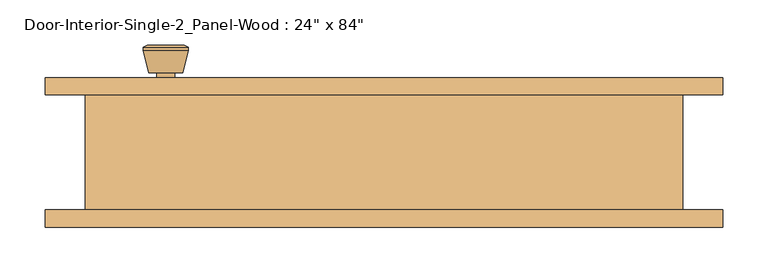
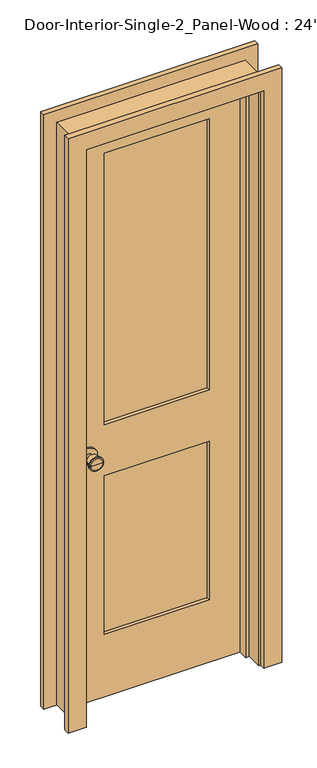
"""IFC4 building model written with IfcOpenShell, lengths in millimetres: door geometry."""

from ifc_helpers import new_model, si_unit, point, frame, frame_2d, origin, place, context, project, spatial, polyline, circle_curve, trimmed, segment, composite_curve, outline, extrude, faceted_brep, source, transform, mapped, element, save
from ifc_brep_helpers import plane_surface, cylinder_surface, revolved_surface, advanced_brep


def door_596d7c92(model_context):
    return source(origin(), model_context, "Body", "SolidModel", [
        advanced_brep(
        [(-241.3, 19.4, 914.4), (-231.3, 19.4, 914.4), (-251.3, 19.4, 914.4), (-220.8241324, -29.6, 914.4), (-241.3, -29.6, 914.4), (-261.7758676, -29.6, 914.4), (-216.3, -27.7721319, 914.4), (-266.3, -27.7721319, 914.4), (-216.3, -24.3084537, 914.4), (-266.3, -24.3084537, 914.4), (-222.663764, 0.4, 914.4), (-259.936236, 0.4, 914.4), (-231.3, 0.4, 914.4), (-251.3, 0.4, 914.4)],
        [
            (0, 1),
            (1, 2, circle_curve(frame((-241.3, 19.4, 914.4), z_axis=(0.0, 1.0, 0.0), x_axis=(-1.0, 0.0, 0.0)), 10.0)),
            (2, 0),
            (2, 1, circle_curve(frame((-241.3, 19.4, 914.4), z_axis=(0.0, 1.0, 0.0), x_axis=(-1.0, 0.0, 0.0)), 10.0)),
            (3, 4),
            (4, 5),
            (5, 3, circle_curve(frame((-241.3, -29.6, 914.4), z_axis=(0.0, -1.0, 0.0), x_axis=(-1.0, 0.0, 0.0)), 20.4758676)),
            (3, 5, circle_curve(frame((-241.3, -29.6, 914.4), z_axis=(0.0, -1.0, 0.0), x_axis=(-1.0, 0.0, 0.0)), 20.4758676)),
            (6, 3),
            (5, 7),
            (7, 6, circle_curve(frame((-241.3, -27.7721319, 914.4), z_axis=(0.0, -1.0, 0.0), x_axis=(-1.0, 0.0, 0.0)), 25.0)),
            (6, 7, circle_curve(frame((-241.3, -27.7721319, 914.4), z_axis=(0.0, -1.0, 0.0), x_axis=(-1.0, 0.0, 0.0)), 25.0)),
            (8, 6),
            (7, 9),
            (9, 8, circle_curve(frame((-241.3, -24.3084537, 914.4), z_axis=(0.0, -1.0, 0.0), x_axis=(-1.0, 0.0, 0.0)), 25.0)),
            (8, 9, circle_curve(frame((-241.3, -24.3084537, 914.4), z_axis=(0.0, -1.0, 0.0), x_axis=(-1.0, 0.0, 0.0)), 25.0)),
            (10, 8),
            (9, 11),
            (11, 10, circle_curve(frame((-241.3, 0.4, 914.4), z_axis=(0.0, -1.0, 0.0), x_axis=(-1.0, 0.0, 0.0)), 18.636236)),
            (10, 11, circle_curve(frame((-241.3, 0.4, 914.4), z_axis=(0.0, -1.0, 0.0), x_axis=(-1.0, 0.0, 0.0)), 18.636236)),
            (12, 10),
            (11, 13),
            (13, 12, circle_curve(frame((-241.3, 0.4, 914.4), z_axis=(0.0, -1.0, 0.0), x_axis=(-1.0, 0.0, 0.0)), 10.0)),
            (12, 13, circle_curve(frame((-241.3, 0.4, 914.4), z_axis=(0.0, -1.0, 0.0), x_axis=(-1.0, 0.0, 0.0)), 10.0)),
            (1, 12),
            (13, 2),
        ],
        [
            plane_surface(frame((-241.3, 19.4, 914.4), z_axis=(0.0, 1.0, 0.0), x_axis=(-1.0, 0.0, 0.0))),
            plane_surface(frame((-241.3, -29.6, 914.4), z_axis=(0.0, -1.0, 0.0), x_axis=(-1.0, 0.0, 0.0))),
            revolved_surface(polyline([(-261.7758676, -29.6, 914.4), (-266.3, -27.7721319, 914.4)]), (-241.3, 19.4, 914.4), (0.0, 1.0, 0.0)),
            cylinder_surface(frame((-241.3, 19.4, 914.4), z_axis=(0.0, 1.0, 0.0), x_axis=(-1.0, 0.0, 0.0)), 25.0),
            revolved_surface(polyline([(-266.3, -24.3084537, 914.4), (-259.936236, 0.4, 914.4)]), (-241.3, 19.4, 914.4), (0.0, 1.0, 0.0)),
            plane_surface(frame((-241.3, 0.4, 914.4), z_axis=(0.0, 1.0, 0.0), x_axis=(-1.0, 0.0, 0.0))),
            cylinder_surface(frame((-241.3, 19.4, 914.4), z_axis=(0.0, 1.0, 0.0), x_axis=(-1.0, 0.0, 0.0)), 10.0),
        ],
        [
            (0, [[1, 2, 3]]),
            (0, [[-3, 4, -1]]),
            (1, [[5, 6, 7]]),
            (1, [[-6, -5, 8]]),
            (2, [[9, -7, 10, 11]]),
            (2, [[-10, -8, -9, 12]]),
            (3, [[13, -11, 14, 15]]),
            (3, [[-14, -12, -13, 16]]),
            (4, [[17, -15, 18, 19]]),
            (4, [[-18, -16, -17, 20]]),
            (5, [[21, -19, 22, 23]]),
            (5, [[-22, -20, -21, 24]]),
            (6, [[25, -23, 26, -2]]),
            (6, [[-26, -24, -25, -4]]),
        ],
    ),
        extrude(outline(composite_curve([segment(trimmed(circle_curve(frame_2d((914.4, -241.3)), 30.0), [point((914.4, -271.3))], [point((914.4, -211.3))], False, "CARTESIAN"), True, "CONTINUOUS"), segment(trimmed(circle_curve(frame_2d((914.4, -241.3)), 30.0), [point((914.4, -211.3))], [point((914.4, -271.3))], False, "CARTESIAN"), True, "CONTINUOUS")], self_intersect=False)), frame((0.0, 19.4, 0.0), z_axis=(0.0, 1.0, 0.0), x_axis=(0.0, 0.0, 1.0)), (0.0, 0.0, 1.0), 6.0),
        advanced_brep(
        [(-241.3, 66.325, 914.4), (-251.3, 66.325, 914.4), (-231.3, 66.325, 914.4), (-220.8241324, 115.325, 914.4), (-261.7758676, 115.325, 914.4), (-241.3, 115.325, 914.4), (-216.3, 113.4971319, 914.4), (-266.3, 113.4971319, 914.4), (-216.3, 110.0334537, 914.4), (-266.3, 110.0334537, 914.4), (-222.663764, 85.325, 914.4), (-259.936236, 85.325, 914.4), (-231.3, 85.325, 914.4), (-251.3, 85.325, 914.4)],
        [
            (0, 1),
            (1, 2, circle_curve(frame((-241.3, 66.325, 914.4), z_axis=(0.0, -1.0, 0.0), x_axis=(-1.0, 0.0, 0.0)), 10.0)),
            (2, 0),
            (2, 1, circle_curve(frame((-241.3, 66.325, 914.4), z_axis=(0.0, -1.0, 0.0), x_axis=(-1.0, 0.0, 0.0)), 10.0)),
            (3, 4, circle_curve(frame((-241.3, 115.325, 914.4), z_axis=(0.0, 1.0, 0.0), x_axis=(-1.0, 0.0, 0.0)), 20.4758676)),
            (4, 5),
            (5, 3),
            (4, 3, circle_curve(frame((-241.3, 115.325, 914.4), z_axis=(0.0, 1.0, 0.0), x_axis=(-1.0, 0.0, 0.0)), 20.4758676)),
            (6, 7, circle_curve(frame((-241.3, 113.4971319, 914.4), z_axis=(0.0, 1.0, 0.0), x_axis=(-1.0, 0.0, 0.0)), 25.0)),
            (7, 4),
            (3, 6),
            (7, 6, circle_curve(frame((-241.3, 113.4971319, 914.4), z_axis=(0.0, 1.0, 0.0), x_axis=(-1.0, 0.0, 0.0)), 25.0)),
            (8, 9, circle_curve(frame((-241.3, 110.0334537, 914.4), z_axis=(0.0, 1.0, 0.0), x_axis=(-1.0, 0.0, 0.0)), 25.0)),
            (9, 7),
            (6, 8),
            (9, 8, circle_curve(frame((-241.3, 110.0334537, 914.4), z_axis=(0.0, 1.0, 0.0), x_axis=(-1.0, 0.0, 0.0)), 25.0)),
            (10, 11, circle_curve(frame((-241.3, 85.325, 914.4), z_axis=(0.0, 1.0, 0.0), x_axis=(-1.0, 0.0, 0.0)), 18.636236)),
            (11, 9),
            (8, 10),
            (11, 10, circle_curve(frame((-241.3, 85.325, 914.4), z_axis=(0.0, 1.0, 0.0), x_axis=(-1.0, 0.0, 0.0)), 18.636236)),
            (12, 13, circle_curve(frame((-241.3, 85.325, 914.4), z_axis=(0.0, 1.0, 0.0), x_axis=(-1.0, 0.0, 0.0)), 10.0)),
            (13, 11),
            (10, 12),
            (13, 12, circle_curve(frame((-241.3, 85.325, 914.4), z_axis=(0.0, 1.0, 0.0), x_axis=(-1.0, 0.0, 0.0)), 10.0)),
            (1, 13),
            (12, 2),
        ],
        [
            plane_surface(frame((-241.3, 66.325, 914.4), z_axis=(0.0, -1.0, 0.0), x_axis=(-1.0, 0.0, 0.0))),
            plane_surface(frame((-241.3, 115.325, 914.4), z_axis=(0.0, 1.0, 0.0), x_axis=(-1.0, 0.0, 0.0))),
            revolved_surface(polyline([(-261.7758676, 115.325, 914.4), (-266.3, 113.4971319, 914.4)]), (-241.3, 66.325, 914.4), (0.0, -1.0, 0.0)),
            cylinder_surface(frame((-241.3, 66.325, 914.4), z_axis=(0.0, -1.0, 0.0), x_axis=(-1.0, 0.0, 0.0)), 25.0),
            revolved_surface(polyline([(-266.3, 110.0334537, 914.4), (-259.936236, 85.325, 914.4)]), (-241.3, 66.325, 914.4), (0.0, -1.0, 0.0)),
            plane_surface(frame((-241.3, 85.325, 914.4), z_axis=(0.0, -1.0, 0.0), x_axis=(-1.0, 0.0, 0.0))),
            cylinder_surface(frame((-241.3, 66.325, 914.4), z_axis=(0.0, -1.0, 0.0), x_axis=(-1.0, 0.0, 0.0)), 10.0),
        ],
        [
            (0, [[1, 2, 3]]),
            (0, [[-3, 4, -1]]),
            (1, [[5, 6, 7]]),
            (1, [[8, -7, -6]]),
            (2, [[9, 10, -5, 11]]),
            (2, [[12, -11, -8, -10]]),
            (3, [[13, 14, -9, 15]]),
            (3, [[16, -15, -12, -14]]),
            (4, [[17, 18, -13, 19]]),
            (4, [[20, -19, -16, -18]]),
            (5, [[21, 22, -17, 23]]),
            (5, [[24, -23, -20, -22]]),
            (6, [[-2, 25, -21, 26]]),
            (6, [[-4, -26, -24, -25]]),
        ],
    ),
        extrude(outline(composite_curve([segment(trimmed(circle_curve(frame_2d((914.4, -241.3)), 30.0), [point((914.4, -271.3))], [point((914.4, -211.3))], False, "CARTESIAN"), True, "CONTINUOUS"), segment(trimmed(circle_curve(frame_2d((914.4, -241.3)), 30.0), [point((914.4, -211.3))], [point((914.4, -271.3))], False, "CARTESIAN"), True, "CONTINUOUS")], self_intersect=False)), frame((0.0, 60.325, 0.0), z_axis=(0.0, 1.0, 0.0), x_axis=(0.0, 0.0, 1.0)), (0.0, 0.0, 1.0), 6.0),
        faceted_brep([(330.2, 60.325, 0.0), (330.2, -66.675, 0.0), (304.8, -66.675, 0.0), (304.8, -9.525, 0.0), (292.1, -9.525, 0.0), (292.1, 25.4, 0.0), (304.8, 25.4, 0.0), (304.8, 60.325, 0.0), (330.2, 60.325, 2159.0), (330.2, -66.675, 2159.0), (-330.2, -66.675, 2159.0), (-330.2, -66.675, 0.0), (-304.8, -66.675, 0.0), (-304.8, -66.675, 2133.6), (304.8, -66.675, 2133.6), (304.8, -9.525, 2133.6), (-304.8, -9.525, 2133.6), (-304.8, -9.525, 0.0), (-292.1, -9.525, 0.0), (-292.1, -9.525, 2120.9), (292.1, -9.525, 2120.9), (292.1, 25.4, 2120.9), (-292.1, 25.4, 2120.9), (-292.1, 25.4, 0.0), (-304.8, 25.4, 0.0), (-304.8, 25.4, 2133.6), (304.8, 25.4, 2133.6), (304.8, 60.325, 2133.6), (-304.8, 60.325, 2133.6), (-304.8, 60.325, 0.0), (-330.2, 60.325, 0.0), (-330.2, 60.325, 2159.0)], [[[0, 1, 2, 3, 4, 5, 6, 7]], [[1, 0, 8, 9]], [[2, 1, 9, 10, 11, 12, 13, 14]], [[3, 2, 14, 15]], [[4, 3, 15, 16, 17, 18, 19, 20]], [[5, 4, 20, 21]], [[6, 5, 21, 22, 23, 24, 25, 26]], [[7, 6, 26, 27]], [[0, 7, 27, 28, 29, 30, 31, 8]], [[9, 8, 31, 10]], [[15, 14, 13, 16]], [[21, 20, 19, 22]], [[27, 26, 25, 28]], [[30, 29, 24, 23, 18, 17, 12, 11]], [[10, 31, 30, 11]], [[16, 13, 12, 17]], [[22, 19, 18, 23]], [[28, 25, 24, 29]]]),
        extrude(outline(polyline([(2133.6, -304.8), (0.0, -304.8), (0.0, 304.8), (2133.6, 304.8), (2133.6, -304.8)]), holes=[polyline([(2014.5375, -184.15), (2014.5375, 184.15), (1009.65, 184.15), (1009.65, -184.15), (2014.5375, -184.15)]), polyline([(819.15, -184.15), (819.15, 184.15), (231.775, 184.15), (231.775, -184.15), (819.15, -184.15)])]), frame((0.0, 25.4, 0.0), z_axis=(0.0, 1.0, 0.0), x_axis=(0.0, 0.0, 1.0)), (0.0, 0.0, 1.0), 34.925),
        extrude(outline(polyline([(184.15, 37.0416667), (-184.15, 37.0416667), (-184.15, 48.6833333), (184.15, 48.6833333), (184.15, 37.0416667)])), frame((0.0, 0.0, 1009.65), z_axis=(0.0, 0.0, 1.0), x_axis=(1.0, 0.0, 0.0)), (0.0, 0.0, 1.0), 1004.8875),
        extrude(outline(polyline([(184.15, 37.0416667), (-184.15, 37.0416667), (-184.15, 48.6833333), (184.15, 48.6833333), (184.15, 37.0416667)])), frame((0.0, 0.0, 231.775), z_axis=(0.0, 0.0, 1.0), x_axis=(1.0, 0.0, 0.0)), (0.0, 0.0, 1.0), 587.375),
        extrude(outline(polyline([(0.0, 311.15), (0.0, 374.65), (2203.45, 374.65), (2203.45, -374.65), (0.0, -374.65), (0.0, -311.15), (2139.95, -311.15), (2139.95, 311.15), (0.0, 311.15)])), frame((0.0, 60.325, 0.0), z_axis=(0.0, 1.0, 0.0), x_axis=(0.0, 0.0, 1.0)), (0.0, 0.0, 1.0), 19.05),
        extrude(outline(polyline([(0.0, 311.15), (0.0, 374.65), (2203.45, 374.65), (2203.45, -374.65), (0.0, -374.65), (0.0, -311.15), (2139.95, -311.15), (2139.95, 311.15), (0.0, 311.15)])), frame((0.0, -85.725, 0.0), z_axis=(0.0, 1.0, 0.0), x_axis=(0.0, 0.0, 1.0)), (0.0, 0.0, 1.0), 19.05),
    ])


if __name__ == "__main__":
    model = new_model("IFC4")
    model_context = context("Model", 3, world=origin())
    ifc_project = project(units=[si_unit("LENGTHUNIT", "METRE", prefix="MILLI")], contexts=[model_context])
    site = spatial("IfcSite", under=ifc_project)
    building = spatial("IfcBuilding", under=site)
    placement = place(None, origin())
    door_shape = door_596d7c92(model_context)
    element("IfcDoor", 1, ObjectType="Door-Interior-Single-2_Panel-Wood : 24\" x 84\"", at=placement, inside=building, context=model_context, shape_type="MappedRepresentation", body=[
        mapped(door_shape, transform((0.0, 0.0, 0.0), x_axis=(1.0, 0.0, 0.0), y_axis=(0.0, 1.0, 0.0), z_axis=(0.0, 0.0, 1.0))),
    ])
    save(model, "model.ifc")

# Revit data of these elements
# Type "Door-Interior-Single-2_Panel-Wood : 24\" x 84\""
#   Type Mark = "10"
#   Assembly Code = "C1020300"
#   Analytic Construction = "Wooden"
#   Top Rail = 0' - 4 11/16"
#   Thickness = 0' - 1 3/8"
#   Thermal Resistance (R) = 2.5876 (h·ft²·°F)/BTU
#   Swing Angle [instance default] = 90.00°
#   Stiles = 0' - 4 3/4"
#   Rough Width = 2' - 2"
#   Rough Height = 7' - 1"
#   Lock Rail = 0' - 7 1/2"
#   Height = 7' - 0"
#   Width = 2' - 0"
#   Heat Transfer Coefficient (U) = 0.3865 BTU/(h·ft²·°F)
#   Bottom Rail = 0' - 9 1/8"
#   Trim Material = Cherry
#   Panel Material = Cherry
#   Frame Material = Cherry
#   Door Handle Material = Aluminum
#   Visual Light Transmittance = 0
#   Solar Heat Gain Coefficient = 0
#   Wall Closure = (empty or 0)
#   Function = (empty or 0)
# Element 1 (IfcDoor, "Door-Interior-Single-2_Panel-Wood : 24\" x 84\"")
#   Materials on its faces: "Cherry", "Aluminum"
# Materials
#   "Cherry": class "Wood", colour RGB 226 177 128, transparency 0, Description = "Prunus Serotina", Cost = 0
#   "Aluminum": class "Metal", colour RGB 247 247 247, transparency 0, Description = "Aluminum 6061", Cost = 0
